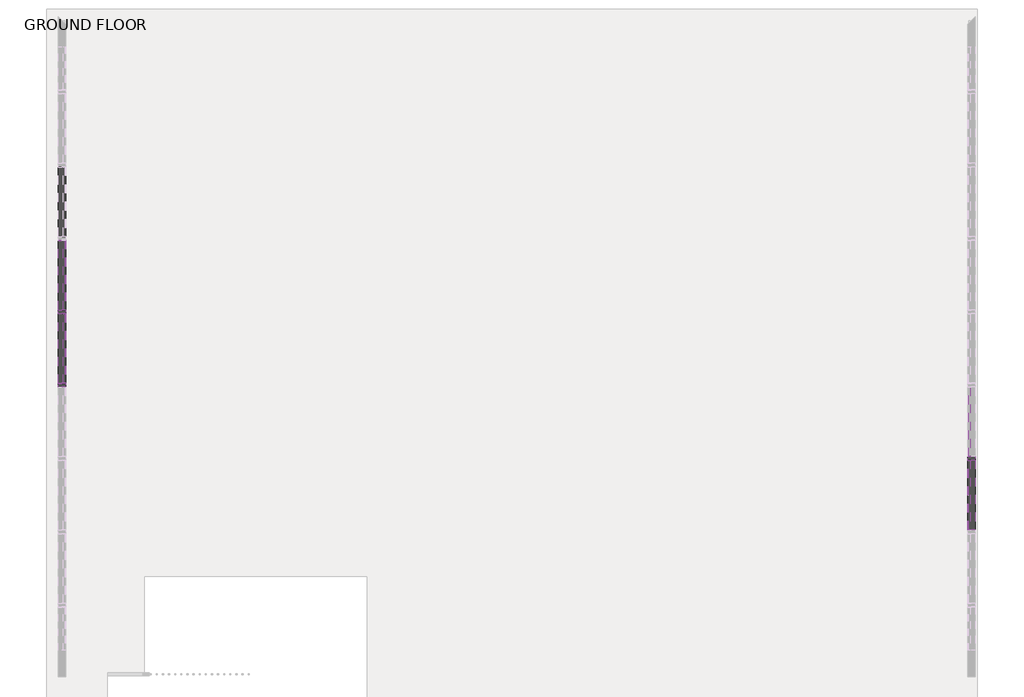
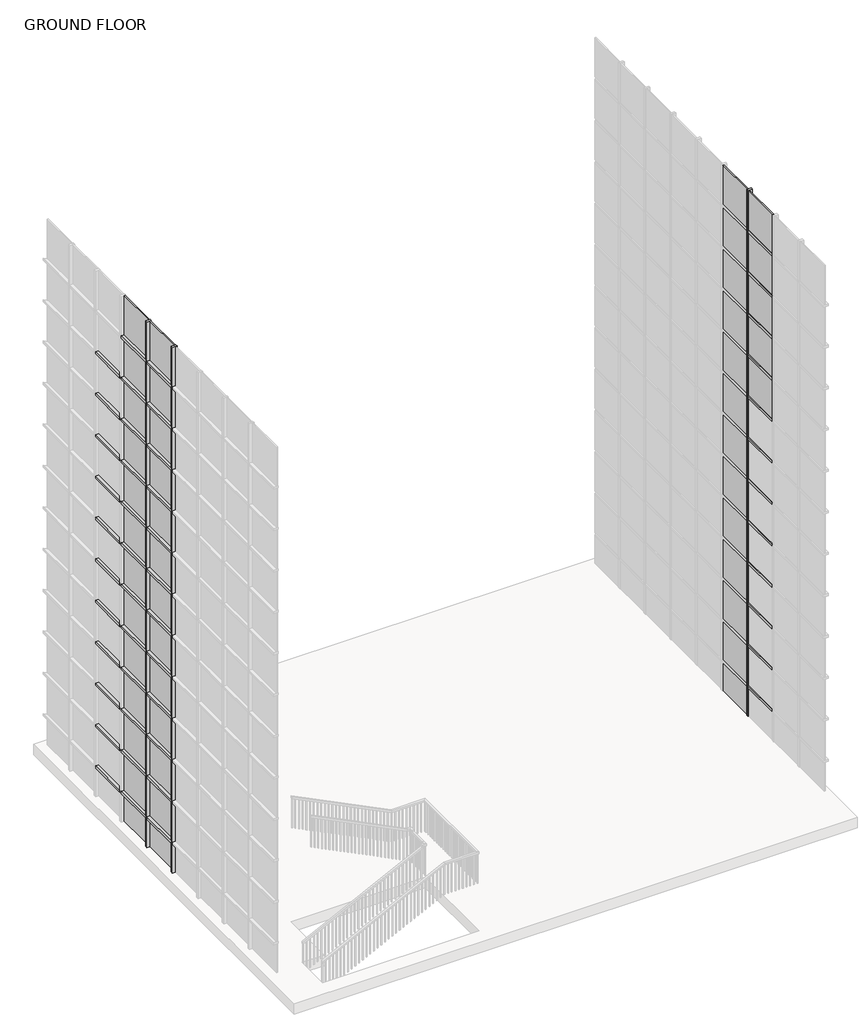
# One storey, part 7 of 16: 86 members, 44 plates.
"""IFC4 building model written with IfcOpenShell, lengths in millimetres."""

from ifc_helpers import new_model, si_unit, origin, place, context, project, spatial, transform, mapped, element, save
from components import member_b860638c, member_31fee25f, member_49b1bc66, system_panel_glazed_49652e9e

model = new_model("IFC4")

# Units and contexts
model_context = context("Model", 3, world=origin())
ifc_project = project(units=[si_unit("LENGTHUNIT", "METRE", prefix="MILLI")], contexts=[model_context])

# Site, building, storey
site = spatial("IfcSite", under=ifc_project)
building = spatial("IfcBuilding", under=site)
storey = spatial("IfcBuildingStorey", under=building, Name="GROUND FLOOR", Elevation=0.0)

# Members
placement = place(None, origin())
member_shape = member_b860638c(model_context)
element("IfcMember", 1, ObjectType="Rectangular Mullion : 2.5\" x 5\" rectangular", at=placement, inside=storey, context=model_context, shape_type="MappedRepresentation", body=[
    mapped(member_shape, transform((5962.6982466, -901.7938032, 0.0), x_axis=(0.0, 1.0, 0.0), y_axis=(1.0, 0.0, 0.0), z_axis=(0.0, 0.0, -1.0))),
])
element("IfcMember", 2, ObjectType="Rectangular Mullion : 2.5\" x 5\" rectangular", at=placement, inside=storey, context=model_context, shape_type="MappedRepresentation", body=[
    mapped(member_shape, transform((-9124.9017534, 1532.7961967, 0.0), x_axis=(0.0, -1.0, 0.0), y_axis=(-1.0, 0.0, 0.0), z_axis=(0.0, 0.0, -1.0))),
])
element("IfcMember", 3, ObjectType="Rectangular Mullion : 2.5\" x 5\" rectangular", at=placement, inside=storey, context=model_context, shape_type="MappedRepresentation", body=[
    mapped(member_shape, transform((-9124.9017534, 315.5011968, 0.0), x_axis=(0.0, -1.0, 0.0), y_axis=(-1.0, 0.0, 0.0), z_axis=(0.0, 0.0, -1.0))),
])
member_2_shape = member_31fee25f(model_context)
element("IfcMember", 4, ObjectType="Rectangular Mullion : 2.5\" x 5\" rectangular", at=placement, inside=storey, context=model_context, shape_type="MappedRepresentation", body=[
    mapped(member_2_shape, transform((5962.6982466, -901.7938032, 1168.8884615), x_axis=(0.0, 1.0, 0.0), y_axis=(1.0, 0.0, 0.0), z_axis=(0.0, 0.0, -1.0))),
])
element("IfcMember", 5, ObjectType="Rectangular Mullion : 2.5\" x 5\" rectangular", at=placement, inside=storey, context=model_context, shape_type="MappedRepresentation", body=[
    mapped(member_2_shape, transform((5962.6982466, -901.7938032, 2369.5269231), x_axis=(0.0, 1.0, 0.0), y_axis=(1.0, 0.0, 0.0), z_axis=(0.0, 0.0, -1.0))),
])
element("IfcMember", 6, ObjectType="Rectangular Mullion : 2.5\" x 5\" rectangular", at=placement, inside=storey, context=model_context, shape_type="MappedRepresentation", body=[
    mapped(member_2_shape, transform((5962.6982466, -901.7938032, 3570.1653846), x_axis=(0.0, 1.0, 0.0), y_axis=(1.0, 0.0, 0.0), z_axis=(0.0, 0.0, -1.0))),
])
element("IfcMember", 7, ObjectType="Rectangular Mullion : 2.5\" x 5\" rectangular", at=placement, inside=storey, context=model_context, shape_type="MappedRepresentation", body=[
    mapped(member_2_shape, transform((5962.6982466, -901.7938032, 4770.8038462), x_axis=(0.0, 1.0, 0.0), y_axis=(1.0, 0.0, 0.0), z_axis=(0.0, 0.0, -1.0))),
])
element("IfcMember", 8, ObjectType="Rectangular Mullion : 2.5\" x 5\" rectangular", at=placement, inside=storey, context=model_context, shape_type="MappedRepresentation", body=[
    mapped(member_2_shape, transform((5962.6982466, -901.7938032, 5971.4423077), x_axis=(0.0, 1.0, 0.0), y_axis=(1.0, 0.0, 0.0), z_axis=(0.0, 0.0, -1.0))),
])
element("IfcMember", 9, ObjectType="Rectangular Mullion : 2.5\" x 5\" rectangular", at=placement, inside=storey, context=model_context, shape_type="MappedRepresentation", body=[
    mapped(member_2_shape, transform((5962.6982466, -901.7938032, 7172.0807692), x_axis=(0.0, 1.0, 0.0), y_axis=(1.0, 0.0, 0.0), z_axis=(0.0, 0.0, -1.0))),
])
element("IfcMember", 10, ObjectType="Rectangular Mullion : 2.5\" x 5\" rectangular", at=placement, inside=storey, context=model_context, shape_type="MappedRepresentation", body=[
    mapped(member_2_shape, transform((5962.6982466, -901.7938032, 8372.7192308), x_axis=(0.0, 1.0, 0.0), y_axis=(1.0, 0.0, 0.0), z_axis=(0.0, 0.0, -1.0))),
])
element("IfcMember", 11, ObjectType="Rectangular Mullion : 2.5\" x 5\" rectangular", at=placement, inside=storey, context=model_context, shape_type="MappedRepresentation", body=[
    mapped(member_2_shape, transform((5962.6982466, -901.7938032, 9573.3576923), x_axis=(0.0, 1.0, 0.0), y_axis=(1.0, 0.0, 0.0), z_axis=(0.0, 0.0, -1.0))),
])
element("IfcMember", 12, ObjectType="Rectangular Mullion : 2.5\" x 5\" rectangular", at=placement, inside=storey, context=model_context, shape_type="MappedRepresentation", body=[
    mapped(member_2_shape, transform((5962.6982466, -901.7938032, 10773.9961538), x_axis=(0.0, 1.0, 0.0), y_axis=(1.0, 0.0, 0.0), z_axis=(0.0, 0.0, -1.0))),
])
element("IfcMember", 13, ObjectType="Rectangular Mullion : 2.5\" x 5\" rectangular", at=placement, inside=storey, context=model_context, shape_type="MappedRepresentation", body=[
    mapped(member_2_shape, transform((5962.6982466, -901.7938032, 11974.6346154), x_axis=(0.0, 1.0, 0.0), y_axis=(1.0, 0.0, 0.0), z_axis=(0.0, 0.0, -1.0))),
])
element("IfcMember", 14, ObjectType="Rectangular Mullion : 2.5\" x 5\" rectangular", at=placement, inside=storey, context=model_context, shape_type="MappedRepresentation", body=[
    mapped(member_2_shape, transform((5962.6982466, -901.7938032, 13175.2730769), x_axis=(0.0, 1.0, 0.0), y_axis=(1.0, 0.0, 0.0), z_axis=(0.0, 0.0, -1.0))),
])
element("IfcMember", 15, ObjectType="Rectangular Mullion : 2.5\" x 5\" rectangular", at=placement, inside=storey, context=model_context, shape_type="MappedRepresentation", body=[
    mapped(member_2_shape, transform((-9124.9017534, 1532.7961967, 1168.8884615), x_axis=(0.0, -1.0, 0.0), y_axis=(-1.0, 0.0, 0.0), z_axis=(0.0, 0.0, -1.0))),
])
element("IfcMember", 16, ObjectType="Rectangular Mullion : 2.5\" x 5\" rectangular", at=placement, inside=storey, context=model_context, shape_type="MappedRepresentation", body=[
    mapped(member_2_shape, transform((-9124.9017534, 315.5011968, 1168.8884615), x_axis=(0.0, -1.0, 0.0), y_axis=(-1.0, 0.0, 0.0), z_axis=(0.0, 0.0, -1.0))),
])
element("IfcMember", 17, ObjectType="Rectangular Mullion : 2.5\" x 5\" rectangular", at=placement, inside=storey, context=model_context, shape_type="MappedRepresentation", body=[
    mapped(member_2_shape, transform((-9124.9017534, 1532.7961967, 2369.5269231), x_axis=(0.0, -1.0, 0.0), y_axis=(-1.0, 0.0, 0.0), z_axis=(0.0, 0.0, -1.0))),
])
element("IfcMember", 18, ObjectType="Rectangular Mullion : 2.5\" x 5\" rectangular", at=placement, inside=storey, context=model_context, shape_type="MappedRepresentation", body=[
    mapped(member_2_shape, transform((-9124.9017534, 315.5011968, 2369.5269231), x_axis=(0.0, -1.0, 0.0), y_axis=(-1.0, 0.0, 0.0), z_axis=(0.0, 0.0, -1.0))),
])
element("IfcMember", 19, ObjectType="Rectangular Mullion : 2.5\" x 5\" rectangular", at=placement, inside=storey, context=model_context, shape_type="MappedRepresentation", body=[
    mapped(member_2_shape, transform((-9124.9017534, 1532.7961967, 3570.1653846), x_axis=(0.0, -1.0, 0.0), y_axis=(-1.0, 0.0, 0.0), z_axis=(0.0, 0.0, -1.0))),
])
element("IfcMember", 20, ObjectType="Rectangular Mullion : 2.5\" x 5\" rectangular", at=placement, inside=storey, context=model_context, shape_type="MappedRepresentation", body=[
    mapped(member_2_shape, transform((-9124.9017534, 315.5011968, 3570.1653846), x_axis=(0.0, -1.0, 0.0), y_axis=(-1.0, 0.0, 0.0), z_axis=(0.0, 0.0, -1.0))),
])
element("IfcMember", 21, ObjectType="Rectangular Mullion : 2.5\" x 5\" rectangular", at=placement, inside=storey, context=model_context, shape_type="MappedRepresentation", body=[
    mapped(member_2_shape, transform((-9124.9017534, 1532.7961967, 4770.8038462), x_axis=(0.0, -1.0, 0.0), y_axis=(-1.0, 0.0, 0.0), z_axis=(0.0, 0.0, -1.0))),
])
element("IfcMember", 22, ObjectType="Rectangular Mullion : 2.5\" x 5\" rectangular", at=placement, inside=storey, context=model_context, shape_type="MappedRepresentation", body=[
    mapped(member_2_shape, transform((-9124.9017534, 315.5011968, 4770.8038462), x_axis=(0.0, -1.0, 0.0), y_axis=(-1.0, 0.0, 0.0), z_axis=(0.0, 0.0, -1.0))),
])
element("IfcMember", 23, ObjectType="Rectangular Mullion : 2.5\" x 5\" rectangular", at=placement, inside=storey, context=model_context, shape_type="MappedRepresentation", body=[
    mapped(member_2_shape, transform((-9124.9017534, 1532.7961967, 5971.4423077), x_axis=(0.0, -1.0, 0.0), y_axis=(-1.0, 0.0, 0.0), z_axis=(0.0, 0.0, -1.0))),
])
element("IfcMember", 24, ObjectType="Rectangular Mullion : 2.5\" x 5\" rectangular", at=placement, inside=storey, context=model_context, shape_type="MappedRepresentation", body=[
    mapped(member_2_shape, transform((-9124.9017534, 315.5011968, 5971.4423077), x_axis=(0.0, -1.0, 0.0), y_axis=(-1.0, 0.0, 0.0), z_axis=(0.0, 0.0, -1.0))),
])
element("IfcMember", 25, ObjectType="Rectangular Mullion : 2.5\" x 5\" rectangular", at=placement, inside=storey, context=model_context, shape_type="MappedRepresentation", body=[
    mapped(member_2_shape, transform((-9124.9017534, 1532.7961967, 7172.0807692), x_axis=(0.0, -1.0, 0.0), y_axis=(-1.0, 0.0, 0.0), z_axis=(0.0, 0.0, -1.0))),
])
element("IfcMember", 26, ObjectType="Rectangular Mullion : 2.5\" x 5\" rectangular", at=placement, inside=storey, context=model_context, shape_type="MappedRepresentation", body=[
    mapped(member_2_shape, transform((-9124.9017534, 315.5011968, 7172.0807692), x_axis=(0.0, -1.0, 0.0), y_axis=(-1.0, 0.0, 0.0), z_axis=(0.0, 0.0, -1.0))),
])
element("IfcMember", 27, ObjectType="Rectangular Mullion : 2.5\" x 5\" rectangular", at=placement, inside=storey, context=model_context, shape_type="MappedRepresentation", body=[
    mapped(member_2_shape, transform((-9124.9017534, 1532.7961967, 8372.7192308), x_axis=(0.0, -1.0, 0.0), y_axis=(-1.0, 0.0, 0.0), z_axis=(0.0, 0.0, -1.0))),
])
element("IfcMember", 28, ObjectType="Rectangular Mullion : 2.5\" x 5\" rectangular", at=placement, inside=storey, context=model_context, shape_type="MappedRepresentation", body=[
    mapped(member_2_shape, transform((-9124.9017534, 315.5011968, 8372.7192308), x_axis=(0.0, -1.0, 0.0), y_axis=(-1.0, 0.0, 0.0), z_axis=(0.0, 0.0, -1.0))),
])
element("IfcMember", 29, ObjectType="Rectangular Mullion : 2.5\" x 5\" rectangular", at=placement, inside=storey, context=model_context, shape_type="MappedRepresentation", body=[
    mapped(member_2_shape, transform((-9124.9017534, 1532.7961967, 9573.3576923), x_axis=(0.0, -1.0, 0.0), y_axis=(-1.0, 0.0, 0.0), z_axis=(0.0, 0.0, -1.0))),
])
element("IfcMember", 30, ObjectType="Rectangular Mullion : 2.5\" x 5\" rectangular", at=placement, inside=storey, context=model_context, shape_type="MappedRepresentation", body=[
    mapped(member_2_shape, transform((-9124.9017534, 315.5011968, 9573.3576923), x_axis=(0.0, -1.0, 0.0), y_axis=(-1.0, 0.0, 0.0), z_axis=(0.0, 0.0, -1.0))),
])
element("IfcMember", 31, ObjectType="Rectangular Mullion : 2.5\" x 5\" rectangular", at=placement, inside=storey, context=model_context, shape_type="MappedRepresentation", body=[
    mapped(member_2_shape, transform((-9124.9017534, 1532.7961967, 10773.9961538), x_axis=(0.0, -1.0, 0.0), y_axis=(-1.0, 0.0, 0.0), z_axis=(0.0, 0.0, -1.0))),
])
element("IfcMember", 32, ObjectType="Rectangular Mullion : 2.5\" x 5\" rectangular", at=placement, inside=storey, context=model_context, shape_type="MappedRepresentation", body=[
    mapped(member_2_shape, transform((-9124.9017534, 315.5011968, 10773.9961538), x_axis=(0.0, -1.0, 0.0), y_axis=(-1.0, 0.0, 0.0), z_axis=(0.0, 0.0, -1.0))),
])
element("IfcMember", 33, ObjectType="Rectangular Mullion : 2.5\" x 5\" rectangular", at=placement, inside=storey, context=model_context, shape_type="MappedRepresentation", body=[
    mapped(member_2_shape, transform((-9124.9017534, 1532.7961967, 11974.6346154), x_axis=(0.0, -1.0, 0.0), y_axis=(-1.0, 0.0, 0.0), z_axis=(0.0, 0.0, -1.0))),
])
element("IfcMember", 34, ObjectType="Rectangular Mullion : 2.5\" x 5\" rectangular", at=placement, inside=storey, context=model_context, shape_type="MappedRepresentation", body=[
    mapped(member_2_shape, transform((-9124.9017534, 315.5011968, 11974.6346154), x_axis=(0.0, -1.0, 0.0), y_axis=(-1.0, 0.0, 0.0), z_axis=(0.0, 0.0, -1.0))),
])
element("IfcMember", 35, ObjectType="Rectangular Mullion : 2.5\" x 5\" rectangular", at=placement, inside=storey, context=model_context, shape_type="MappedRepresentation", body=[
    mapped(member_2_shape, transform((-9124.9017534, 1532.7961967, 13175.2730769), x_axis=(0.0, -1.0, 0.0), y_axis=(-1.0, 0.0, 0.0), z_axis=(0.0, 0.0, -1.0))),
])
element("IfcMember", 36, ObjectType="Rectangular Mullion : 2.5\" x 5\" rectangular", at=placement, inside=storey, context=model_context, shape_type="MappedRepresentation", body=[
    mapped(member_2_shape, transform((-9124.9017534, 315.5011968, 13175.2730769), x_axis=(0.0, -1.0, 0.0), y_axis=(-1.0, 0.0, 0.0), z_axis=(0.0, 0.0, -1.0))),
])
element("IfcMember", 37, ObjectType="Rectangular Mullion : 2.5\" x 5\" rectangular", at=placement, inside=storey, context=model_context, shape_type="MappedRepresentation", body=[
    mapped(member_shape, transform((5962.6982466, -901.7938032, 14375.9115385), x_axis=(0.0, 1.0, 0.0), y_axis=(1.0, 0.0, 0.0), z_axis=(0.0, 0.0, -1.0))),
])
element("IfcMember", 38, ObjectType="Rectangular Mullion : 2.5\" x 5\" rectangular", at=placement, inside=storey, context=model_context, shape_type="MappedRepresentation", body=[
    mapped(member_shape, transform((-9124.9017534, 1532.7961967, 14375.9115385), x_axis=(0.0, -1.0, 0.0), y_axis=(-1.0, 0.0, 0.0), z_axis=(0.0, 0.0, -1.0))),
])
element("IfcMember", 39, ObjectType="Rectangular Mullion : 2.5\" x 5\" rectangular", at=placement, inside=storey, context=model_context, shape_type="MappedRepresentation", body=[
    mapped(member_shape, transform((-9124.9017534, 315.5011968, 14375.9115385), x_axis=(0.0, -1.0, 0.0), y_axis=(-1.0, 0.0, 0.0), z_axis=(0.0, 0.0, -1.0))),
])
member_3_shape = member_49b1bc66(model_context)
element("IfcMember", 40, ObjectType="Rectangular Mullion : 2.5\" x 5\" rectangular", at=placement, inside=storey, context=model_context, shape_type="MappedRepresentation", body=[
    mapped(member_3_shape, transform((5962.6982466, -933.5438032, 1168.8884615), x_axis=(0.0, 0.0, 1.0), y_axis=(1.0, 0.0, 0.0), z_axis=(0.0, 1.0, 0.0))),
])
element("IfcMember", 41, ObjectType="Rectangular Mullion : 2.5\" x 5\" rectangular", at=placement, inside=storey, context=model_context, shape_type="MappedRepresentation", body=[
    mapped(member_3_shape, transform((5962.6982466, -933.5438032, 2369.5269231), x_axis=(0.0, 0.0, 1.0), y_axis=(1.0, 0.0, 0.0), z_axis=(0.0, 1.0, 0.0))),
])
element("IfcMember", 42, ObjectType="Rectangular Mullion : 2.5\" x 5\" rectangular", at=placement, inside=storey, context=model_context, shape_type="MappedRepresentation", body=[
    mapped(member_3_shape, transform((5962.6982466, -933.5438032, 3570.1653846), x_axis=(0.0, 0.0, 1.0), y_axis=(1.0, 0.0, 0.0), z_axis=(0.0, 1.0, 0.0))),
])
element("IfcMember", 43, ObjectType="Rectangular Mullion : 2.5\" x 5\" rectangular", at=placement, inside=storey, context=model_context, shape_type="MappedRepresentation", body=[
    mapped(member_3_shape, transform((5962.6982466, -933.5438032, 4770.8038462), x_axis=(0.0, 0.0, 1.0), y_axis=(1.0, 0.0, 0.0), z_axis=(0.0, 1.0, 0.0))),
])
element("IfcMember", 44, ObjectType="Rectangular Mullion : 2.5\" x 5\" rectangular", at=placement, inside=storey, context=model_context, shape_type="MappedRepresentation", body=[
    mapped(member_3_shape, transform((5962.6982466, -933.5438032, 5971.4423077), x_axis=(0.0, 0.0, 1.0), y_axis=(1.0, 0.0, 0.0), z_axis=(0.0, 1.0, 0.0))),
])
element("IfcMember", 45, ObjectType="Rectangular Mullion : 2.5\" x 5\" rectangular", at=placement, inside=storey, context=model_context, shape_type="MappedRepresentation", body=[
    mapped(member_3_shape, transform((5962.6982466, -933.5438032, 7172.0807692), x_axis=(0.0, 0.0, 1.0), y_axis=(1.0, 0.0, 0.0), z_axis=(0.0, 1.0, 0.0))),
])
element("IfcMember", 46, ObjectType="Rectangular Mullion : 2.5\" x 5\" rectangular", at=placement, inside=storey, context=model_context, shape_type="MappedRepresentation", body=[
    mapped(member_3_shape, transform((5962.6982466, -933.5438032, 8372.7192308), x_axis=(0.0, 0.0, 1.0), y_axis=(1.0, 0.0, 0.0), z_axis=(0.0, 1.0, 0.0))),
])
element("IfcMember", 47, ObjectType="Rectangular Mullion : 2.5\" x 5\" rectangular", at=placement, inside=storey, context=model_context, shape_type="MappedRepresentation", body=[
    mapped(member_3_shape, transform((5962.6982466, -933.5438032, 9573.3576923), x_axis=(0.0, 0.0, 1.0), y_axis=(1.0, 0.0, 0.0), z_axis=(0.0, 1.0, 0.0))),
])
element("IfcMember", 48, ObjectType="Rectangular Mullion : 2.5\" x 5\" rectangular", at=placement, inside=storey, context=model_context, shape_type="MappedRepresentation", body=[
    mapped(member_3_shape, transform((5962.6982466, -933.5438032, 10773.9961538), x_axis=(0.0, 0.0, 1.0), y_axis=(1.0, 0.0, 0.0), z_axis=(0.0, 1.0, 0.0))),
])
element("IfcMember", 49, ObjectType="Rectangular Mullion : 2.5\" x 5\" rectangular", at=placement, inside=storey, context=model_context, shape_type="MappedRepresentation", body=[
    mapped(member_3_shape, transform((5962.6982466, -933.5438032, 11974.6346154), x_axis=(0.0, 0.0, 1.0), y_axis=(1.0, 0.0, 0.0), z_axis=(0.0, 1.0, 0.0))),
])
element("IfcMember", 50, ObjectType="Rectangular Mullion : 2.5\" x 5\" rectangular", at=placement, inside=storey, context=model_context, shape_type="MappedRepresentation", body=[
    mapped(member_3_shape, transform((5962.6982466, -933.5438032, 13175.2730769), x_axis=(0.0, 0.0, 1.0), y_axis=(1.0, 0.0, 0.0), z_axis=(0.0, 1.0, 0.0))),
])
element("IfcMember", 51, ObjectType="Rectangular Mullion : 2.5\" x 5\" rectangular", at=placement, inside=storey, context=model_context, shape_type="MappedRepresentation", body=[
    mapped(member_3_shape, transform((5962.6982466, -933.5438032, 14375.9115385), x_axis=(0.0, 0.0, 1.0), y_axis=(1.0, 0.0, 0.0), z_axis=(0.0, 1.0, 0.0))),
])
element("IfcMember", 52, ObjectType="Rectangular Mullion : 2.5\" x 5\" rectangular", at=placement, inside=storey, context=model_context, shape_type="MappedRepresentation", body=[
    mapped(member_3_shape, transform((-9124.9017534, 2781.8411967, 1168.8884615), x_axis=(0.0, 0.0, 1.0), y_axis=(-1.0, 0.0, 0.0), z_axis=(0.0, -1.0, 0.0))),
])
element("IfcMember", 53, ObjectType="Rectangular Mullion : 2.5\" x 5\" rectangular", at=placement, inside=storey, context=model_context, shape_type="MappedRepresentation", body=[
    mapped(member_3_shape, transform((-9124.9017534, 1564.5461967, 1168.8884615), x_axis=(0.0, 0.0, 1.0), y_axis=(-1.0, 0.0, 0.0), z_axis=(0.0, -1.0, 0.0))),
])
element("IfcMember", 54, ObjectType="Rectangular Mullion : 2.5\" x 5\" rectangular", at=placement, inside=storey, context=model_context, shape_type="MappedRepresentation", body=[
    mapped(member_3_shape, transform((-9124.9017534, 347.2511968, 1168.8884615), x_axis=(0.0, 0.0, 1.0), y_axis=(-1.0, 0.0, 0.0), z_axis=(0.0, -1.0, 0.0))),
])
element("IfcMember", 55, ObjectType="Rectangular Mullion : 2.5\" x 5\" rectangular", at=placement, inside=storey, context=model_context, shape_type="MappedRepresentation", body=[
    mapped(member_3_shape, transform((-9124.9017534, 2781.8411967, 2369.5269231), x_axis=(0.0, 0.0, 1.0), y_axis=(-1.0, 0.0, 0.0), z_axis=(0.0, -1.0, 0.0))),
])
element("IfcMember", 56, ObjectType="Rectangular Mullion : 2.5\" x 5\" rectangular", at=placement, inside=storey, context=model_context, shape_type="MappedRepresentation", body=[
    mapped(member_3_shape, transform((-9124.9017534, 1564.5461967, 2369.5269231), x_axis=(0.0, 0.0, 1.0), y_axis=(-1.0, 0.0, 0.0), z_axis=(0.0, -1.0, 0.0))),
])
element("IfcMember", 57, ObjectType="Rectangular Mullion : 2.5\" x 5\" rectangular", at=placement, inside=storey, context=model_context, shape_type="MappedRepresentation", body=[
    mapped(member_3_shape, transform((-9124.9017534, 347.2511968, 2369.5269231), x_axis=(0.0, 0.0, 1.0), y_axis=(-1.0, 0.0, 0.0), z_axis=(0.0, -1.0, 0.0))),
])
element("IfcMember", 58, ObjectType="Rectangular Mullion : 2.5\" x 5\" rectangular", at=placement, inside=storey, context=model_context, shape_type="MappedRepresentation", body=[
    mapped(member_3_shape, transform((-9124.9017534, 2781.8411967, 3570.1653846), x_axis=(0.0, 0.0, 1.0), y_axis=(-1.0, 0.0, 0.0), z_axis=(0.0, -1.0, 0.0))),
])
element("IfcMember", 59, ObjectType="Rectangular Mullion : 2.5\" x 5\" rectangular", at=placement, inside=storey, context=model_context, shape_type="MappedRepresentation", body=[
    mapped(member_3_shape, transform((-9124.9017534, 1564.5461967, 3570.1653846), x_axis=(0.0, 0.0, 1.0), y_axis=(-1.0, 0.0, 0.0), z_axis=(0.0, -1.0, 0.0))),
])
element("IfcMember", 60, ObjectType="Rectangular Mullion : 2.5\" x 5\" rectangular", at=placement, inside=storey, context=model_context, shape_type="MappedRepresentation", body=[
    mapped(member_3_shape, transform((-9124.9017534, 347.2511968, 3570.1653846), x_axis=(0.0, 0.0, 1.0), y_axis=(-1.0, 0.0, 0.0), z_axis=(0.0, -1.0, 0.0))),
])
element("IfcMember", 61, ObjectType="Rectangular Mullion : 2.5\" x 5\" rectangular", at=placement, inside=storey, context=model_context, shape_type="MappedRepresentation", body=[
    mapped(member_3_shape, transform((-9124.9017534, 2781.8411967, 4770.8038462), x_axis=(0.0, 0.0, 1.0), y_axis=(-1.0, 0.0, 0.0), z_axis=(0.0, -1.0, 0.0))),
])
element("IfcMember", 62, ObjectType="Rectangular Mullion : 2.5\" x 5\" rectangular", at=placement, inside=storey, context=model_context, shape_type="MappedRepresentation", body=[
    mapped(member_3_shape, transform((-9124.9017534, 1564.5461967, 4770.8038462), x_axis=(0.0, 0.0, 1.0), y_axis=(-1.0, 0.0, 0.0), z_axis=(0.0, -1.0, 0.0))),
])
element("IfcMember", 63, ObjectType="Rectangular Mullion : 2.5\" x 5\" rectangular", at=placement, inside=storey, context=model_context, shape_type="MappedRepresentation", body=[
    mapped(member_3_shape, transform((-9124.9017534, 347.2511968, 4770.8038462), x_axis=(0.0, 0.0, 1.0), y_axis=(-1.0, 0.0, 0.0), z_axis=(0.0, -1.0, 0.0))),
])
element("IfcMember", 64, ObjectType="Rectangular Mullion : 2.5\" x 5\" rectangular", at=placement, inside=storey, context=model_context, shape_type="MappedRepresentation", body=[
    mapped(member_3_shape, transform((-9124.9017534, 2781.8411967, 5971.4423077), x_axis=(0.0, 0.0, 1.0), y_axis=(-1.0, 0.0, 0.0), z_axis=(0.0, -1.0, 0.0))),
])
element("IfcMember", 65, ObjectType="Rectangular Mullion : 2.5\" x 5\" rectangular", at=placement, inside=storey, context=model_context, shape_type="MappedRepresentation", body=[
    mapped(member_3_shape, transform((-9124.9017534, 1564.5461967, 5971.4423077), x_axis=(0.0, 0.0, 1.0), y_axis=(-1.0, 0.0, 0.0), z_axis=(0.0, -1.0, 0.0))),
])
element("IfcMember", 66, ObjectType="Rectangular Mullion : 2.5\" x 5\" rectangular", at=placement, inside=storey, context=model_context, shape_type="MappedRepresentation", body=[
    mapped(member_3_shape, transform((-9124.9017534, 347.2511968, 5971.4423077), x_axis=(0.0, 0.0, 1.0), y_axis=(-1.0, 0.0, 0.0), z_axis=(0.0, -1.0, 0.0))),
])
element("IfcMember", 67, ObjectType="Rectangular Mullion : 2.5\" x 5\" rectangular", at=placement, inside=storey, context=model_context, shape_type="MappedRepresentation", body=[
    mapped(member_3_shape, transform((-9124.9017534, 2781.8411967, 7172.0807692), x_axis=(0.0, 0.0, 1.0), y_axis=(-1.0, 0.0, 0.0), z_axis=(0.0, -1.0, 0.0))),
])
element("IfcMember", 68, ObjectType="Rectangular Mullion : 2.5\" x 5\" rectangular", at=placement, inside=storey, context=model_context, shape_type="MappedRepresentation", body=[
    mapped(member_3_shape, transform((-9124.9017534, 1564.5461967, 7172.0807692), x_axis=(0.0, 0.0, 1.0), y_axis=(-1.0, 0.0, 0.0), z_axis=(0.0, -1.0, 0.0))),
])
element("IfcMember", 69, ObjectType="Rectangular Mullion : 2.5\" x 5\" rectangular", at=placement, inside=storey, context=model_context, shape_type="MappedRepresentation", body=[
    mapped(member_3_shape, transform((-9124.9017534, 347.2511968, 7172.0807692), x_axis=(0.0, 0.0, 1.0), y_axis=(-1.0, 0.0, 0.0), z_axis=(0.0, -1.0, 0.0))),
])
element("IfcMember", 70, ObjectType="Rectangular Mullion : 2.5\" x 5\" rectangular", at=placement, inside=storey, context=model_context, shape_type="MappedRepresentation", body=[
    mapped(member_3_shape, transform((-9124.9017534, 2781.8411967, 8372.7192308), x_axis=(0.0, 0.0, 1.0), y_axis=(-1.0, 0.0, 0.0), z_axis=(0.0, -1.0, 0.0))),
])
element("IfcMember", 71, ObjectType="Rectangular Mullion : 2.5\" x 5\" rectangular", at=placement, inside=storey, context=model_context, shape_type="MappedRepresentation", body=[
    mapped(member_3_shape, transform((-9124.9017534, 1564.5461967, 8372.7192308), x_axis=(0.0, 0.0, 1.0), y_axis=(-1.0, 0.0, 0.0), z_axis=(0.0, -1.0, 0.0))),
])
element("IfcMember", 72, ObjectType="Rectangular Mullion : 2.5\" x 5\" rectangular", at=placement, inside=storey, context=model_context, shape_type="MappedRepresentation", body=[
    mapped(member_3_shape, transform((-9124.9017534, 347.2511968, 8372.7192308), x_axis=(0.0, 0.0, 1.0), y_axis=(-1.0, 0.0, 0.0), z_axis=(0.0, -1.0, 0.0))),
])
element("IfcMember", 73, ObjectType="Rectangular Mullion : 2.5\" x 5\" rectangular", at=placement, inside=storey, context=model_context, shape_type="MappedRepresentation", body=[
    mapped(member_3_shape, transform((-9124.9017534, 2781.8411967, 9573.3576923), x_axis=(0.0, 0.0, 1.0), y_axis=(-1.0, 0.0, 0.0), z_axis=(0.0, -1.0, 0.0))),
])
element("IfcMember", 74, ObjectType="Rectangular Mullion : 2.5\" x 5\" rectangular", at=placement, inside=storey, context=model_context, shape_type="MappedRepresentation", body=[
    mapped(member_3_shape, transform((-9124.9017534, 1564.5461967, 9573.3576923), x_axis=(0.0, 0.0, 1.0), y_axis=(-1.0, 0.0, 0.0), z_axis=(0.0, -1.0, 0.0))),
])
element("IfcMember", 75, ObjectType="Rectangular Mullion : 2.5\" x 5\" rectangular", at=placement, inside=storey, context=model_context, shape_type="MappedRepresentation", body=[
    mapped(member_3_shape, transform((-9124.9017534, 347.2511968, 9573.3576923), x_axis=(0.0, 0.0, 1.0), y_axis=(-1.0, 0.0, 0.0), z_axis=(0.0, -1.0, 0.0))),
])
element("IfcMember", 76, ObjectType="Rectangular Mullion : 2.5\" x 5\" rectangular", at=placement, inside=storey, context=model_context, shape_type="MappedRepresentation", body=[
    mapped(member_3_shape, transform((-9124.9017534, 2781.8411967, 10773.9961538), x_axis=(0.0, 0.0, 1.0), y_axis=(-1.0, 0.0, 0.0), z_axis=(0.0, -1.0, 0.0))),
])
element("IfcMember", 77, ObjectType="Rectangular Mullion : 2.5\" x 5\" rectangular", at=placement, inside=storey, context=model_context, shape_type="MappedRepresentation", body=[
    mapped(member_3_shape, transform((-9124.9017534, 1564.5461967, 10773.9961538), x_axis=(0.0, 0.0, 1.0), y_axis=(-1.0, 0.0, 0.0), z_axis=(0.0, -1.0, 0.0))),
])
element("IfcMember", 78, ObjectType="Rectangular Mullion : 2.5\" x 5\" rectangular", at=placement, inside=storey, context=model_context, shape_type="MappedRepresentation", body=[
    mapped(member_3_shape, transform((-9124.9017534, 347.2511968, 10773.9961538), x_axis=(0.0, 0.0, 1.0), y_axis=(-1.0, 0.0, 0.0), z_axis=(0.0, -1.0, 0.0))),
])
element("IfcMember", 79, ObjectType="Rectangular Mullion : 2.5\" x 5\" rectangular", at=placement, inside=storey, context=model_context, shape_type="MappedRepresentation", body=[
    mapped(member_3_shape, transform((-9124.9017534, 2781.8411967, 11974.6346154), x_axis=(0.0, 0.0, 1.0), y_axis=(-1.0, 0.0, 0.0), z_axis=(0.0, -1.0, 0.0))),
])
element("IfcMember", 80, ObjectType="Rectangular Mullion : 2.5\" x 5\" rectangular", at=placement, inside=storey, context=model_context, shape_type="MappedRepresentation", body=[
    mapped(member_3_shape, transform((-9124.9017534, 1564.5461967, 11974.6346154), x_axis=(0.0, 0.0, 1.0), y_axis=(-1.0, 0.0, 0.0), z_axis=(0.0, -1.0, 0.0))),
])
element("IfcMember", 81, ObjectType="Rectangular Mullion : 2.5\" x 5\" rectangular", at=placement, inside=storey, context=model_context, shape_type="MappedRepresentation", body=[
    mapped(member_3_shape, transform((-9124.9017534, 347.2511968, 11974.6346154), x_axis=(0.0, 0.0, 1.0), y_axis=(-1.0, 0.0, 0.0), z_axis=(0.0, -1.0, 0.0))),
])
element("IfcMember", 82, ObjectType="Rectangular Mullion : 2.5\" x 5\" rectangular", at=placement, inside=storey, context=model_context, shape_type="MappedRepresentation", body=[
    mapped(member_3_shape, transform((-9124.9017534, 2781.8411967, 13175.2730769), x_axis=(0.0, 0.0, 1.0), y_axis=(-1.0, 0.0, 0.0), z_axis=(0.0, -1.0, 0.0))),
])
element("IfcMember", 83, ObjectType="Rectangular Mullion : 2.5\" x 5\" rectangular", at=placement, inside=storey, context=model_context, shape_type="MappedRepresentation", body=[
    mapped(member_3_shape, transform((-9124.9017534, 1564.5461967, 13175.2730769), x_axis=(0.0, 0.0, 1.0), y_axis=(-1.0, 0.0, 0.0), z_axis=(0.0, -1.0, 0.0))),
])
element("IfcMember", 84, ObjectType="Rectangular Mullion : 2.5\" x 5\" rectangular", at=placement, inside=storey, context=model_context, shape_type="MappedRepresentation", body=[
    mapped(member_3_shape, transform((-9124.9017534, 347.2511968, 13175.2730769), x_axis=(0.0, 0.0, 1.0), y_axis=(-1.0, 0.0, 0.0), z_axis=(0.0, -1.0, 0.0))),
])
element("IfcMember", 85, ObjectType="Rectangular Mullion : 2.5\" x 5\" rectangular", at=placement, inside=storey, context=model_context, shape_type="MappedRepresentation", body=[
    mapped(member_3_shape, transform((-9124.9017534, 1564.5461967, 14375.9115385), x_axis=(0.0, 0.0, 1.0), y_axis=(-1.0, 0.0, 0.0), z_axis=(0.0, -1.0, 0.0))),
])
element("IfcMember", 86, ObjectType="Rectangular Mullion : 2.5\" x 5\" rectangular", at=placement, inside=storey, context=model_context, shape_type="MappedRepresentation", body=[
    mapped(member_3_shape, transform((-9124.9017534, 347.2511968, 14375.9115385), x_axis=(0.0, 0.0, 1.0), y_axis=(-1.0, 0.0, 0.0), z_axis=(0.0, -1.0, 0.0))),
])

# Plates
system_panel_glazed_shape = system_panel_glazed_49652e9e(model_context)
element("IfcPlate", 87, ObjectType="System Panel : Glazed", at=placement, inside=storey, context=model_context, shape_type="MappedRepresentation", body=[
    mapped(system_panel_glazed_shape, transform((5962.6982466, -293.1463032, 0.0), x_axis=(0.0, 1.0, 0.0), y_axis=(-1.0, 0.0, 0.0), z_axis=(0.0, 0.0, 1.0))),
])
element("IfcPlate", 88, ObjectType="System Panel : Glazed", at=placement, inside=storey, context=model_context, shape_type="MappedRepresentation", body=[
    mapped(system_panel_glazed_shape, transform((5962.6982466, -293.1463032, 1200.6384615), x_axis=(0.0, 1.0, 0.0), y_axis=(-1.0, 0.0, 0.0), z_axis=(0.0, 0.0, 1.0))),
])
element("IfcPlate", 89, ObjectType="System Panel : Glazed", at=placement, inside=storey, context=model_context, shape_type="MappedRepresentation", body=[
    mapped(system_panel_glazed_shape, transform((5962.6982466, -293.1463032, 2401.2769231), x_axis=(0.0, 1.0, 0.0), y_axis=(-1.0, 0.0, 0.0), z_axis=(0.0, 0.0, 1.0))),
])
element("IfcPlate", 90, ObjectType="System Panel : Glazed", at=placement, inside=storey, context=model_context, shape_type="MappedRepresentation", body=[
    mapped(system_panel_glazed_shape, transform((5962.6982466, -293.1463032, 3601.9153846), x_axis=(0.0, 1.0, 0.0), y_axis=(-1.0, 0.0, 0.0), z_axis=(0.0, 0.0, 1.0))),
])
element("IfcPlate", 91, ObjectType="System Panel : Glazed", at=placement, inside=storey, context=model_context, shape_type="MappedRepresentation", body=[
    mapped(system_panel_glazed_shape, transform((5962.6982466, -293.1463032, 4802.5538462), x_axis=(0.0, 1.0, 0.0), y_axis=(-1.0, 0.0, 0.0), z_axis=(0.0, 0.0, 1.0))),
])
element("IfcPlate", 92, ObjectType="System Panel : Glazed", at=placement, inside=storey, context=model_context, shape_type="MappedRepresentation", body=[
    mapped(system_panel_glazed_shape, transform((5962.6982466, -293.1463032, 6003.1923077), x_axis=(0.0, 1.0, 0.0), y_axis=(-1.0, 0.0, 0.0), z_axis=(0.0, 0.0, 1.0))),
])
element("IfcPlate", 93, ObjectType="System Panel : Glazed", at=placement, inside=storey, context=model_context, shape_type="MappedRepresentation", body=[
    mapped(system_panel_glazed_shape, transform((5962.6982466, -293.1463032, 7203.8307692), x_axis=(0.0, 1.0, 0.0), y_axis=(-1.0, 0.0, 0.0), z_axis=(0.0, 0.0, 1.0))),
])
element("IfcPlate", 94, ObjectType="System Panel : Glazed", at=placement, inside=storey, context=model_context, shape_type="MappedRepresentation", body=[
    mapped(system_panel_glazed_shape, transform((5962.6982466, -293.1463032, 8404.4692308), x_axis=(0.0, 1.0, 0.0), y_axis=(-1.0, 0.0, 0.0), z_axis=(0.0, 0.0, 1.0))),
])
element("IfcPlate", 95, ObjectType="System Panel : Glazed", at=placement, inside=storey, context=model_context, shape_type="MappedRepresentation", body=[
    mapped(system_panel_glazed_shape, transform((5962.6982466, -1510.4413031, 9605.1076923), x_axis=(0.0, 1.0, 0.0), y_axis=(-1.0, 0.0, 0.0), z_axis=(0.0, 0.0, 1.0))),
])
element("IfcPlate", 96, ObjectType="System Panel : Glazed", at=placement, inside=storey, context=model_context, shape_type="MappedRepresentation", body=[
    mapped(system_panel_glazed_shape, transform((5962.6982466, -293.1463032, 9605.1076923), x_axis=(0.0, 1.0, 0.0), y_axis=(-1.0, 0.0, 0.0), z_axis=(0.0, 0.0, 1.0))),
])
element("IfcPlate", 97, ObjectType="System Panel : Glazed", at=placement, inside=storey, context=model_context, shape_type="MappedRepresentation", body=[
    mapped(system_panel_glazed_shape, transform((5962.6982466, -1510.4413031, 10805.7461538), x_axis=(0.0, 1.0, 0.0), y_axis=(-1.0, 0.0, 0.0), z_axis=(0.0, 0.0, 1.0))),
])
element("IfcPlate", 98, ObjectType="System Panel : Glazed", at=placement, inside=storey, context=model_context, shape_type="MappedRepresentation", body=[
    mapped(system_panel_glazed_shape, transform((5962.6982466, -293.1463032, 10805.7461538), x_axis=(0.0, 1.0, 0.0), y_axis=(-1.0, 0.0, 0.0), z_axis=(0.0, 0.0, 1.0))),
])
element("IfcPlate", 99, ObjectType="System Panel : Glazed", at=placement, inside=storey, context=model_context, shape_type="MappedRepresentation", body=[
    mapped(system_panel_glazed_shape, transform((5962.6982466, -1510.4413031, 12006.3846154), x_axis=(0.0, 1.0, 0.0), y_axis=(-1.0, 0.0, 0.0), z_axis=(0.0, 0.0, 1.0))),
])
element("IfcPlate", 100, ObjectType="System Panel : Glazed", at=placement, inside=storey, context=model_context, shape_type="MappedRepresentation", body=[
    mapped(system_panel_glazed_shape, transform((5962.6982466, -293.1463032, 12006.3846154), x_axis=(0.0, 1.0, 0.0), y_axis=(-1.0, 0.0, 0.0), z_axis=(0.0, 0.0, 1.0))),
])
element("IfcPlate", 101, ObjectType="System Panel : Glazed", at=placement, inside=storey, context=model_context, shape_type="MappedRepresentation", body=[
    mapped(system_panel_glazed_shape, transform((5962.6982466, -1510.4413031, 13207.0230769), x_axis=(0.0, 1.0, 0.0), y_axis=(-1.0, 0.0, 0.0), z_axis=(0.0, 0.0, 1.0))),
])
element("IfcPlate", 102, ObjectType="System Panel : Glazed", at=placement, inside=storey, context=model_context, shape_type="MappedRepresentation", body=[
    mapped(system_panel_glazed_shape, transform((5962.6982466, -293.1463032, 13207.0230769), x_axis=(0.0, 1.0, 0.0), y_axis=(-1.0, 0.0, 0.0), z_axis=(0.0, 0.0, 1.0))),
])
element("IfcPlate", 103, ObjectType="System Panel : Glazed", at=placement, inside=storey, context=model_context, shape_type="MappedRepresentation", body=[
    mapped(system_panel_glazed_shape, transform((5962.6982466, -1510.4413031, 14407.6615385), x_axis=(0.0, 1.0, 0.0), y_axis=(-1.0, 0.0, 0.0), z_axis=(0.0, 0.0, 1.0))),
])
element("IfcPlate", 104, ObjectType="System Panel : Glazed", at=placement, inside=storey, context=model_context, shape_type="MappedRepresentation", body=[
    mapped(system_panel_glazed_shape, transform((5962.6982466, -293.1463032, 14407.6615385), x_axis=(0.0, 1.0, 0.0), y_axis=(-1.0, 0.0, 0.0), z_axis=(0.0, 0.0, 1.0))),
])
element("IfcPlate", 105, ObjectType="System Panel : Glazed", at=placement, inside=storey, context=model_context, shape_type="MappedRepresentation", body=[
    mapped(system_panel_glazed_shape, transform((-9124.9017534, 2141.4436967, 0.0), x_axis=(0.0, -1.0, 0.0), y_axis=(1.0, 0.0, 0.0), z_axis=(0.0, 0.0, 1.0))),
])
element("IfcPlate", 106, ObjectType="System Panel : Glazed", at=placement, inside=storey, context=model_context, shape_type="MappedRepresentation", body=[
    mapped(system_panel_glazed_shape, transform((-9124.9017534, 924.1486967, 0.0), x_axis=(0.0, -1.0, 0.0), y_axis=(1.0, 0.0, 0.0), z_axis=(0.0, 0.0, 1.0))),
])
element("IfcPlate", 107, ObjectType="System Panel : Glazed", at=placement, inside=storey, context=model_context, shape_type="MappedRepresentation", body=[
    mapped(system_panel_glazed_shape, transform((-9124.9017534, 2141.4436967, 1200.6384615), x_axis=(0.0, -1.0, 0.0), y_axis=(1.0, 0.0, 0.0), z_axis=(0.0, 0.0, 1.0))),
])
element("IfcPlate", 108, ObjectType="System Panel : Glazed", at=placement, inside=storey, context=model_context, shape_type="MappedRepresentation", body=[
    mapped(system_panel_glazed_shape, transform((-9124.9017534, 924.1486967, 1200.6384615), x_axis=(0.0, -1.0, 0.0), y_axis=(1.0, 0.0, 0.0), z_axis=(0.0, 0.0, 1.0))),
])
element("IfcPlate", 109, ObjectType="System Panel : Glazed", at=placement, inside=storey, context=model_context, shape_type="MappedRepresentation", body=[
    mapped(system_panel_glazed_shape, transform((-9124.9017534, 2141.4436967, 2401.2769231), x_axis=(0.0, -1.0, 0.0), y_axis=(1.0, 0.0, 0.0), z_axis=(0.0, 0.0, 1.0))),
])
element("IfcPlate", 110, ObjectType="System Panel : Glazed", at=placement, inside=storey, context=model_context, shape_type="MappedRepresentation", body=[
    mapped(system_panel_glazed_shape, transform((-9124.9017534, 924.1486967, 2401.2769231), x_axis=(0.0, -1.0, 0.0), y_axis=(1.0, 0.0, 0.0), z_axis=(0.0, 0.0, 1.0))),
])
element("IfcPlate", 111, ObjectType="System Panel : Glazed", at=placement, inside=storey, context=model_context, shape_type="MappedRepresentation", body=[
    mapped(system_panel_glazed_shape, transform((-9124.9017534, 2141.4436967, 3601.9153846), x_axis=(0.0, -1.0, 0.0), y_axis=(1.0, 0.0, 0.0), z_axis=(0.0, 0.0, 1.0))),
])
element("IfcPlate", 112, ObjectType="System Panel : Glazed", at=placement, inside=storey, context=model_context, shape_type="MappedRepresentation", body=[
    mapped(system_panel_glazed_shape, transform((-9124.9017534, 924.1486967, 3601.9153846), x_axis=(0.0, -1.0, 0.0), y_axis=(1.0, 0.0, 0.0), z_axis=(0.0, 0.0, 1.0))),
])
element("IfcPlate", 113, ObjectType="System Panel : Glazed", at=placement, inside=storey, context=model_context, shape_type="MappedRepresentation", body=[
    mapped(system_panel_glazed_shape, transform((-9124.9017534, 2141.4436967, 4802.5538462), x_axis=(0.0, -1.0, 0.0), y_axis=(1.0, 0.0, 0.0), z_axis=(0.0, 0.0, 1.0))),
])
element("IfcPlate", 114, ObjectType="System Panel : Glazed", at=placement, inside=storey, context=model_context, shape_type="MappedRepresentation", body=[
    mapped(system_panel_glazed_shape, transform((-9124.9017534, 924.1486967, 4802.5538462), x_axis=(0.0, -1.0, 0.0), y_axis=(1.0, 0.0, 0.0), z_axis=(0.0, 0.0, 1.0))),
])
element("IfcPlate", 115, ObjectType="System Panel : Glazed", at=placement, inside=storey, context=model_context, shape_type="MappedRepresentation", body=[
    mapped(system_panel_glazed_shape, transform((-9124.9017534, 2141.4436967, 6003.1923077), x_axis=(0.0, -1.0, 0.0), y_axis=(1.0, 0.0, 0.0), z_axis=(0.0, 0.0, 1.0))),
])
element("IfcPlate", 116, ObjectType="System Panel : Glazed", at=placement, inside=storey, context=model_context, shape_type="MappedRepresentation", body=[
    mapped(system_panel_glazed_shape, transform((-9124.9017534, 924.1486967, 6003.1923077), x_axis=(0.0, -1.0, 0.0), y_axis=(1.0, 0.0, 0.0), z_axis=(0.0, 0.0, 1.0))),
])
element("IfcPlate", 117, ObjectType="System Panel : Glazed", at=placement, inside=storey, context=model_context, shape_type="MappedRepresentation", body=[
    mapped(system_panel_glazed_shape, transform((-9124.9017534, 2141.4436967, 7203.8307692), x_axis=(0.0, -1.0, 0.0), y_axis=(1.0, 0.0, 0.0), z_axis=(0.0, 0.0, 1.0))),
])
element("IfcPlate", 118, ObjectType="System Panel : Glazed", at=placement, inside=storey, context=model_context, shape_type="MappedRepresentation", body=[
    mapped(system_panel_glazed_shape, transform((-9124.9017534, 924.1486967, 7203.8307692), x_axis=(0.0, -1.0, 0.0), y_axis=(1.0, 0.0, 0.0), z_axis=(0.0, 0.0, 1.0))),
])
element("IfcPlate", 119, ObjectType="System Panel : Glazed", at=placement, inside=storey, context=model_context, shape_type="MappedRepresentation", body=[
    mapped(system_panel_glazed_shape, transform((-9124.9017534, 2141.4436967, 8404.4692308), x_axis=(0.0, -1.0, 0.0), y_axis=(1.0, 0.0, 0.0), z_axis=(0.0, 0.0, 1.0))),
])
element("IfcPlate", 120, ObjectType="System Panel : Glazed", at=placement, inside=storey, context=model_context, shape_type="MappedRepresentation", body=[
    mapped(system_panel_glazed_shape, transform((-9124.9017534, 924.1486967, 8404.4692308), x_axis=(0.0, -1.0, 0.0), y_axis=(1.0, 0.0, 0.0), z_axis=(0.0, 0.0, 1.0))),
])
element("IfcPlate", 121, ObjectType="System Panel : Glazed", at=placement, inside=storey, context=model_context, shape_type="MappedRepresentation", body=[
    mapped(system_panel_glazed_shape, transform((-9124.9017534, 2141.4436967, 9605.1076923), x_axis=(0.0, -1.0, 0.0), y_axis=(1.0, 0.0, 0.0), z_axis=(0.0, 0.0, 1.0))),
])
element("IfcPlate", 122, ObjectType="System Panel : Glazed", at=placement, inside=storey, context=model_context, shape_type="MappedRepresentation", body=[
    mapped(system_panel_glazed_shape, transform((-9124.9017534, 924.1486967, 9605.1076923), x_axis=(0.0, -1.0, 0.0), y_axis=(1.0, 0.0, 0.0), z_axis=(0.0, 0.0, 1.0))),
])
element("IfcPlate", 123, ObjectType="System Panel : Glazed", at=placement, inside=storey, context=model_context, shape_type="MappedRepresentation", body=[
    mapped(system_panel_glazed_shape, transform((-9124.9017534, 2141.4436967, 10805.7461538), x_axis=(0.0, -1.0, 0.0), y_axis=(1.0, 0.0, 0.0), z_axis=(0.0, 0.0, 1.0))),
])
element("IfcPlate", 124, ObjectType="System Panel : Glazed", at=placement, inside=storey, context=model_context, shape_type="MappedRepresentation", body=[
    mapped(system_panel_glazed_shape, transform((-9124.9017534, 924.1486967, 10805.7461538), x_axis=(0.0, -1.0, 0.0), y_axis=(1.0, 0.0, 0.0), z_axis=(0.0, 0.0, 1.0))),
])
element("IfcPlate", 125, ObjectType="System Panel : Glazed", at=placement, inside=storey, context=model_context, shape_type="MappedRepresentation", body=[
    mapped(system_panel_glazed_shape, transform((-9124.9017534, 2141.4436967, 12006.3846154), x_axis=(0.0, -1.0, 0.0), y_axis=(1.0, 0.0, 0.0), z_axis=(0.0, 0.0, 1.0))),
])
element("IfcPlate", 126, ObjectType="System Panel : Glazed", at=placement, inside=storey, context=model_context, shape_type="MappedRepresentation", body=[
    mapped(system_panel_glazed_shape, transform((-9124.9017534, 924.1486967, 12006.3846154), x_axis=(0.0, -1.0, 0.0), y_axis=(1.0, 0.0, 0.0), z_axis=(0.0, 0.0, 1.0))),
])
element("IfcPlate", 127, ObjectType="System Panel : Glazed", at=placement, inside=storey, context=model_context, shape_type="MappedRepresentation", body=[
    mapped(system_panel_glazed_shape, transform((-9124.9017534, 2141.4436967, 13207.0230769), x_axis=(0.0, -1.0, 0.0), y_axis=(1.0, 0.0, 0.0), z_axis=(0.0, 0.0, 1.0))),
])
element("IfcPlate", 128, ObjectType="System Panel : Glazed", at=placement, inside=storey, context=model_context, shape_type="MappedRepresentation", body=[
    mapped(system_panel_glazed_shape, transform((-9124.9017534, 924.1486967, 13207.0230769), x_axis=(0.0, -1.0, 0.0), y_axis=(1.0, 0.0, 0.0), z_axis=(0.0, 0.0, 1.0))),
])
element("IfcPlate", 129, ObjectType="System Panel : Glazed", at=placement, inside=storey, context=model_context, shape_type="MappedRepresentation", body=[
    mapped(system_panel_glazed_shape, transform((-9124.9017534, 2141.4436967, 14407.6615385), x_axis=(0.0, -1.0, 0.0), y_axis=(1.0, 0.0, 0.0), z_axis=(0.0, 0.0, 1.0))),
])
element("IfcPlate", 130, ObjectType="System Panel : Glazed", at=placement, inside=storey, context=model_context, shape_type="MappedRepresentation", body=[
    mapped(system_panel_glazed_shape, transform((-9124.9017534, 924.1486967, 14407.6615385), x_axis=(0.0, -1.0, 0.0), y_axis=(1.0, 0.0, 0.0), z_axis=(0.0, 0.0, 1.0))),
])

save(model, "model.ifc")

# Revit data of these elements
# Type "Rectangular Mullion : 2.5\" x 5\" rectangular"
#   built-in parameter 1007304 = 0.416667 (stored number, unit not read)
#   built-in parameter 1007301 = 0.104167 (stored number, unit not read)
#   built-in parameter 1007300 = 0.104167 (stored number, unit not read)
# Type "System Panel : Glazed"
#   Construction Type Id = "GSP4R"
#   Analytic Construction = "1/8 in Pilkington single glazing"
#   Visual Light Transmittance = 0.9
#   Solar Heat Gain Coefficient = 0.86
#   Heat Transfer Coefficient (U) = 1.18115 BTU/(h·ft²·°F)
#   Define Thermal Properties by = 1
# Elements 1, 2, 3, 4, 5, 6, 7, 8, 9, 10, 11, 12, 13, 14, 15, 16, 17, 18, 19, 20, 21, 22, 23, 24, 25, 26, 27, 28, 29, 30, 31, 32, 33, 34, 35, 36, 37, 38, 39, 40, 41, 42, 43, 44, 45, 46, 47, 48, 49, 50, 51, 52, 53, 54, 55, 56, 57, 58, 59, 60, 61, 62, 63, 64, 65, 66, 67, 68, 69, 70, 71, 72, 73, 74, 75, 76, 77, 78, 79, 80, 81, 82, 83, 84, 85, 86 (IfcMember, "Rectangular Mullion : 2.5\" x 5\" rectangular")
#   Phase Created = New Construction
#   Materials on its faces: "Aluminum"
# Elements 87, 88, 89, 90, 91, 92, 93, 94, 95, 96, 97, 98, 99, 100, 101, 102, 103, 104, 105, 106, 107, 108, 109, 110, 111, 112, 113, 114, 115, 116, 117, 118, 119, 120, 121, 122, 123, 124, 125, 126, 127, 128, 129, 130 (IfcPlate, "System Panel : Glazed")
#   Phase Created = New Construction
#   Materials on its faces: "Glass"
# Materials
#   "Aluminum": class "Metal", colour RGB 247 247 247, transparency 0, Description = "Aluminum 6061", Cost = 0
#   "Glass": class "Glass", colour RGB 0 128 192, transparency 0.75, Description = "Soda Lime Glass", Cost = 0
